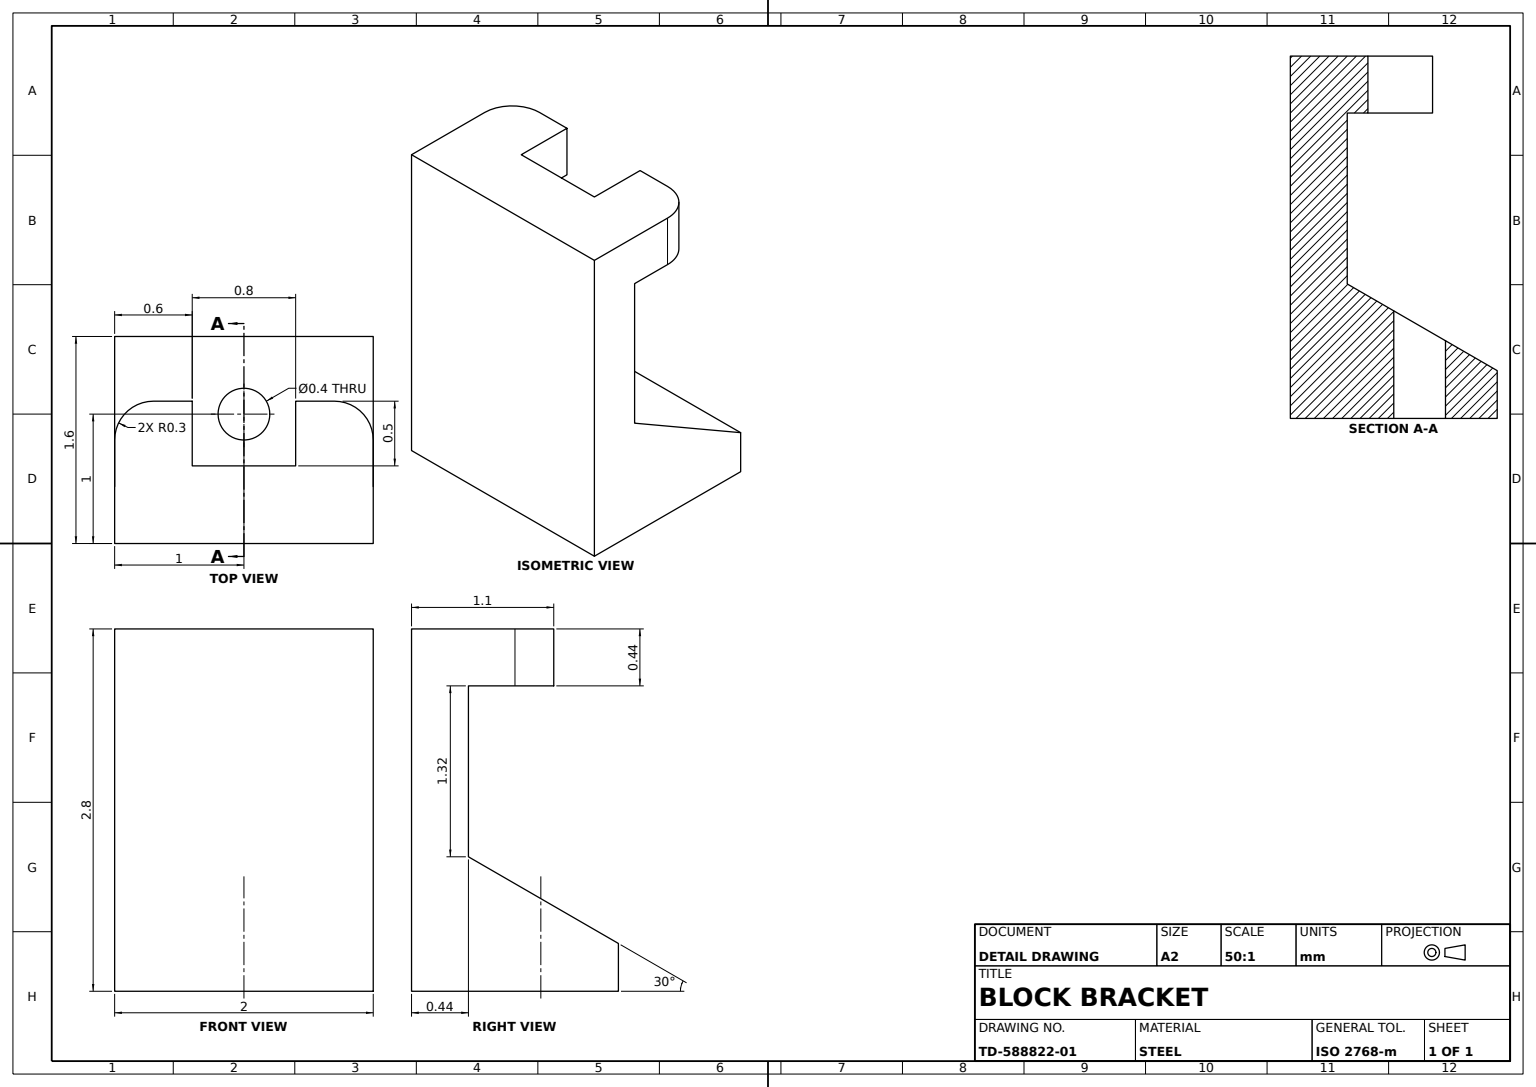
from build123d import *

# Parameters (mm, degrees)
C_BRACKET_BODY_DEPTH         = 2
RECESS_CUT_A_0_44_DEEP_DEPTH = 0.44
RECESS_CUT_B_0_44_DEEP_DEPTH = 0.44
HOLE_SKETCH_R                = 0.2
HOLE_0_4_X_1_DEEP_DEPTH      = 1


with BuildPart() as part:
    # C-Profile Sketch → C-Bracket Body (new body)
    with BuildSketch(Plane.XY):
        Polygon((0, 0), (1.6, 0), (1.6, 2.8), (0.5, 2.8), (0.5, 2.36), (1.16, 2.36), (1.16, 1.039148534), (0, 0.369422221), align=None)
    extrude(amount=-C_BRACKET_BODY_DEPTH)

    # Recess Cut A Sketch → Recess Cut A 0.44 Deep (cut)
    with BuildSketch(Plane(origin=(0, 2.8, 0), x_dir=(1, 0, 0), z_dir=(0, 1, 0))):
        with BuildLine():
            Line((0.5, 2), (0.8, 2))
            ThreePointArc((0.8, 2), (0.587867966, 1.912132034), (0.5, 1.7))
            Line((0.5, 1.7), (0.5, 2))
        make_face()
        with BuildLine():
            Line((0.5, 0), (0.8, 0))
            ThreePointArc((0.8, 0), (0.587867966, 0.087867966), (0.5, 0.3))
            Line((0.5, 0.3), (0.5, 0))
        make_face()
    extrude(amount=-RECESS_CUT_A_0_44_DEEP_DEPTH, mode=Mode.SUBTRACT)

    # Recess Cut B Sketch → Recess Cut B 0.44 Deep (cut)
    with BuildSketch(Plane(origin=(0, 2.8, 0), x_dir=(1, 0, 0), z_dir=(0, 1, 0))):
        Polygon((1, 1), (1, 1.4), (0.5, 1.4), (0.5, 0.6), (1, 0.6), align=None)
    extrude(amount=-RECESS_CUT_B_0_44_DEEP_DEPTH, mode=Mode.SUBTRACT)

    # Hole Sketch → Hole Ø0.4 x 1 Deep (cut)
    with BuildSketch(Plane.XZ):
        with Locations(Location((0.6, -1, 0), (0, 0, 270))):
            Circle(HOLE_SKETCH_R)
    extrude(amount=-HOLE_0_4_X_1_DEEP_DEPTH, mode=Mode.SUBTRACT)


solid = part.part
